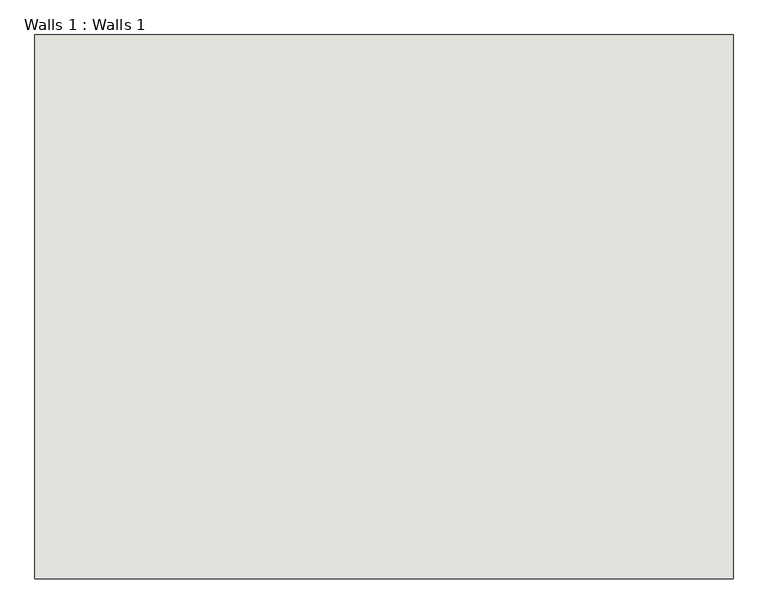
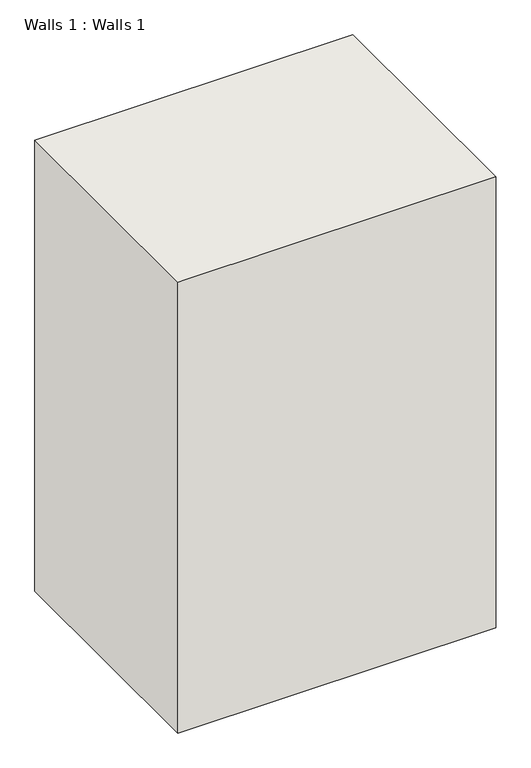
"""IFC4 building model written with IfcOpenShell, lengths in millimetres: wall geometry, Walls 1 : Walls 1."""

from ifc_helpers import new_model, si_unit, frame, origin, place, context, project, spatial, polyline, outline, extrude, source, transform, mapped, element, save


def walls_1_walls_1_d9e15aa8(model_context):
    return source(origin(), model_context, "Body", "SweptSolid", [
        extrude(outline(polyline([(-13671.3981295, 1959.4613684), (-14687.3981295, 1959.4613684), (-14687.3981295, 2750.673096), (-13671.3981295, 2750.673096), (-13671.3981295, 1959.4613684)])), frame((0.0, 0.0, 3235.7023612), z_axis=(0.0, 0.0, 1.0), x_axis=(1.0, 0.0, 0.0)), (0.0, 0.0, 1.0), 1524.0),
    ])


if __name__ == "__main__":
    model = new_model("IFC4")
    model_context = context("Model", 3, world=origin())
    ifc_project = project(units=[si_unit("LENGTHUNIT", "METRE", prefix="MILLI")], contexts=[model_context])
    site = spatial("IfcSite", under=ifc_project)
    building = spatial("IfcBuilding", under=site)
    placement = place(None, origin())
    walls_1_walls_1_shape = walls_1_walls_1_d9e15aa8(model_context)
    element("IfcWall", 1, ObjectType="Walls 1 : Walls 1", at=placement, inside=building, context=model_context, shape_type="MappedRepresentation", body=[
        mapped(walls_1_walls_1_shape, transform((0.0, 0.0, 0.0), x_axis=(1.0, 0.0, 0.0), y_axis=(0.0, 1.0, 0.0), z_axis=(0.0, 0.0, 1.0))),
    ])
    save(model, "model.ifc")

# Revit data of these elements
# Element 1 (IfcWall, "Walls 1 : Walls 1")
#   Materials on its faces: "Default Wall"
# Materials
#   "Default Wall": colour RGB 128 128 128, transparency 0
